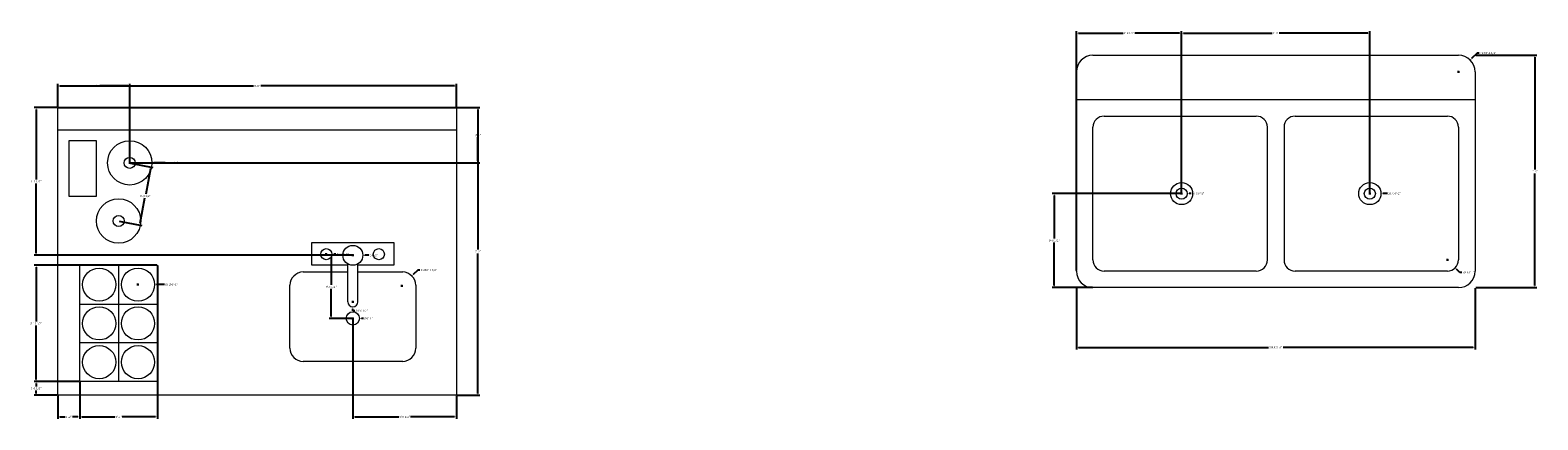
# Model space of a CAD drawing. Units: inches. Extents: x 226 to 1155, y 22 to 494.
# Tile 4 of 7: x 884 to 1020, y 56 to 91. Entities that reach past the tile are written whole.
import ezdxf

# ---------------------------------------------------------------- set-up
doc = ezdxf.new("R2010")
doc.units = ezdxf.units.IN
doc.header["$MEASUREMENT"] = 0
for name, color, linetype, lineweight in [('A-ANNO-DIMS', 2, 'Continuous', 18), ('A-EQPM', 8, 'Continuous', 18), ('A-FLOR-FIXT', 9, 'Continuous', 18)]:
    doc.layers.add(name, color=color, linetype=linetype, lineweight=lineweight)
doc.styles.get("Standard").update_dxf_attribs({"font": 'arial.ttf'})
doc.dimstyles.get("Standard").update_dxf_attribs({"dimtxt": 0.18, "dimasz": 0.18, "dimexe": 0.18, "dimexo": 0.0625, "dimgap": 0.09, "dimtad": 0, "dimtih": 1, "dimtoh": 1, "dimdec": 4, "dimzin": 0, "dimdsep": 46, "dimlunit": 4, "dimtxsty": 'Standard', "dimcen": 0.09, "dimadec": 0, "dimazin": 0, "dimtfac": 1, "dimtdec": 4, "dimtofl": 0, "dimtmove": 0, "dimatfit": 3, "dimfxl": 1, "dimtolj": 1, "dimtzin": 0, "dimarcsym": 0})

# ---------------------------------------------------------------- blocks, each defined once
blk = doc.blocks.new('Sink-double - 36 in top')
for p, q in [((-18, -4), (18, -4)), ((-0.75, -18.5), (-0.75, -6.5)), ((0.75, -6.5), (0.75, -18.5))]:
    blk.add_line(p, q)
for points in [[(-16.5, 0), (16.5, 0)], [(-18, -19.5), (-18, -1.5)], [(18, -1.5), (18, -19.5)], [(-16.5, -18.5), (-16.5, -6.5)], [(-15.5, -5.5), (-1.75, -5.5)], [(1.75, -5.5), (15.5, -5.5)], [(16.5, -6.5), (16.5, -18.5)], [(-1.75, -19.5), (-15.5, -19.5)], [(15.5, -19.5), (1.75, -19.5)], [(16.5, -21), (-16.5, -21)]]:
    blk.add_lwpolyline(points)
for centre, radius in [((-8.5, -12.5), 1), ((-8.5, -12.5), 0.5), ((8.5, -12.5), 1), ((8.5, -12.5), 0.5)]:
    blk.add_circle(centre, radius)
for centre, radius, start, end in [((-16.5, -1.5), 1.5, 90, 180), ((16.5, -1.5), 1.5, 0, 90), ((-15.5, -6.5), 1, 90, 180), ((-1.75, -6.5), 1, 0, 90), ((1.75, -6.5), 1, 90, 180), ((15.5, -6.5), 1, 0, 90), ((-15.5, -18.5), 1, 180, 270), ((-1.75, -18.5), 1, 270, 0), ((1.75, -18.5), 1, 180, 270), ((15.5, -18.5), 1, 270, 0), ((-16.5, -19.5), 1.5, 180, 270), ((16.5, -19.5), 1.5, 270, 0)]:
    blk.add_arc(centre, radius, start, end)
blk = doc.blocks.new('*D52')
at = {"layer": 'A-ANNO-DIMS', "color": 0, "lineweight": -2, "transparency": 16777216}
for p, q in [((978, 67.6), (978, 62.08)), ((1014, 67.6), (1014, 62.08)), ((978.18, 62.26), (995.34, 62.26)), ((1013.82, 62.26), (996.66, 62.26))]:
    blk.add_line(p, q, dxfattribs=at)
at = {"layer": 'A-ANNO-DIMS', "color": 0, "transparency": 16777216}
for points in [[(978.18, 62.29), (978.18, 62.23), (978, 62.26)], [(1013.82, 62.29), (1013.82, 62.23), (1014, 62.26)]]:
    blk.add_solid(points, dxfattribs=at)
at = {"layer": 'Defpoints', "color": 0, "transparency": 16777216}
for p in [(978, 67.66), (1014, 67.66), (1014, 62.26)]:
    blk.add_point(p, dxfattribs=at)
at = {"layer": 'A-ANNO-DIMS', "color": 0, "transparency": 16777216, "insert": (996, 62.26), "char_height": 0.18, "attachment_point": 5}
blk.add_mtext('\\A1;SINK 3\'-0"', dxfattribs=at)
blk = doc.blocks.new('*D53')
at = {"layer": 'A-ANNO-DIMS', "color": 0, "lineweight": -2, "transparency": 16777216}
for p, q in [((1014.06, 88.66), (1019.58, 88.66)), ((1019.4, 88.48), (1019.4, 78.34)), ((1019.4, 67.84), (1019.4, 77.98)), ((1014.06, 67.66), (1019.58, 67.66))]:
    blk.add_line(p, q, dxfattribs=at)
at = {"layer": 'A-ANNO-DIMS', "color": 0, "transparency": 16777216}
for points in [[(1019.37, 88.48), (1019.43, 88.48), (1019.4, 88.66)], [(1019.37, 67.84), (1019.43, 67.84), (1019.4, 67.66)]]:
    blk.add_solid(points, dxfattribs=at)
at = {"layer": 'Defpoints', "color": 0, "transparency": 16777216}
for p in [(1014, 88.66), (1019.4, 88.66), (1014, 67.66)]:
    blk.add_point(p, dxfattribs=at)
at = {"layer": 'A-ANNO-DIMS', "color": 0, "transparency": 16777216, "insert": (1019.4, 78.16), "char_height": 0.18, "attachment_point": 5}
blk.add_mtext('\\A1;1\'-9"', dxfattribs=at)
blk = doc.blocks.new('*D104')
at = {"layer": 'A-ANNO-DIMS', "color": 0, "lineweight": -2, "transparency": 16777216}
for p, q in [((978, 69.22), (978, 90.84)), ((978.18, 90.66), (982.21, 90.66)), ((987.32, 90.66), (983.29, 90.66)), ((987.5, 76.22), (987.5, 90.84))]:
    blk.add_line(p, q, dxfattribs=at)
at = {"layer": 'A-ANNO-DIMS', "color": 0, "transparency": 16777216}
for points in [[(978.18, 90.69), (978.18, 90.63), (978, 90.66)], [(987.32, 90.69), (987.32, 90.63), (987.5, 90.66)]]:
    blk.add_solid(points, dxfattribs=at)
at = {"layer": 'Defpoints', "color": 0, "transparency": 16777216}
for p in [(987.5, 90.66), (987.5, 76.16), (978, 69.16)]:
    blk.add_point(p, dxfattribs=at)
at = {"layer": 'A-ANNO-DIMS', "color": 0, "transparency": 16777216, "insert": (982.75, 90.66), "char_height": 0.18, "attachment_point": 5}
blk.add_mtext('\\A1;0\'-9 1/2"', dxfattribs=at)
blk = doc.blocks.new('*D105')
at = {"layer": 'A-ANNO-DIMS', "color": 0, "lineweight": -2, "transparency": 16777216}
for p, q in [((987.5, 76.22), (987.5, 90.84)), ((987.68, 90.66), (995.68, 90.66)), ((1004.32, 90.66), (996.32, 90.66)), ((1004.5, 76.22), (1004.5, 90.84))]:
    blk.add_line(p, q, dxfattribs=at)
at = {"layer": 'A-ANNO-DIMS', "color": 0, "transparency": 16777216}
for points in [[(987.68, 90.69), (987.68, 90.63), (987.5, 90.66)], [(1004.32, 90.69), (1004.32, 90.63), (1004.5, 90.66)]]:
    blk.add_solid(points, dxfattribs=at)
at = {"layer": 'Defpoints', "color": 0, "transparency": 16777216}
for p in [(1004.5, 90.66), (987.5, 76.16), (1004.5, 76.16)]:
    blk.add_point(p, dxfattribs=at)
at = {"layer": 'A-ANNO-DIMS', "color": 0, "transparency": 16777216, "insert": (996, 90.66), "char_height": 0.18, "attachment_point": 5}
blk.add_mtext('\\A1;1\'-5"', dxfattribs=at)
blk = doc.blocks.new('*D106')
at = {"layer": 'A-ANNO-DIMS', "color": 0, "lineweight": -2, "transparency": 16777216}
for p, q in [((987.44, 76.16), (975.82, 76.16)), ((976, 75.98), (976, 72.09)), ((976, 67.84), (976, 71.73)), ((979.44, 67.66), (975.82, 67.66))]:
    blk.add_line(p, q, dxfattribs=at)
at = {"layer": 'A-ANNO-DIMS', "color": 0, "transparency": 16777216}
for points in [[(975.97, 75.98), (976.03, 75.98), (976, 76.16)], [(975.97, 67.84), (976.03, 67.84), (976, 67.66)]]:
    blk.add_solid(points, dxfattribs=at)
at = {"layer": 'Defpoints', "color": 0, "transparency": 16777216}
for p in [(976, 76.16), (987.5, 76.16), (979.5, 67.66)]:
    blk.add_point(p, dxfattribs=at)
at = {"layer": 'A-ANNO-DIMS', "color": 0, "transparency": 16777216, "insert": (976, 71.91), "char_height": 0.18, "attachment_point": 5}
blk.add_mtext('\\A1;0\'-8 1/2"', dxfattribs=at)
blk = doc.blocks.new('*D107')
at = {"layer": 'A-ANNO-DIMS', "color": 0, "lineweight": -2, "transparency": 16777216}
for p, q in [((886.01, 83.99), (886.01, 86.06)), ((886.19, 85.88), (903.68, 85.88)), ((921.83, 85.88), (904.34, 85.88)), ((922.01, 83.99), (922.01, 86.06))]:
    blk.add_line(p, q, dxfattribs=at)
at = {"layer": 'A-ANNO-DIMS', "color": 0, "transparency": 16777216}
for points in [[(886.19, 85.91), (886.19, 85.85), (886.01, 85.88)], [(921.83, 85.91), (921.83, 85.85), (922.01, 85.88)]]:
    blk.add_solid(points, dxfattribs=at)
at = {"layer": 'Defpoints', "color": 0, "transparency": 16777216}
for p in [(922.01, 85.88), (886.01, 83.93), (922.01, 83.93)]:
    blk.add_point(p, dxfattribs=at)
at = {"layer": 'A-ANNO-DIMS', "color": 0, "transparency": 16777216, "insert": (904.01, 85.88), "char_height": 0.18, "attachment_point": 5}
blk.add_mtext('\\A1;3\'-0"', dxfattribs=at)
blk = doc.blocks.new('*D108')
at = {"layer": 'A-ANNO-DIMS', "color": 0, "lineweight": -2, "transparency": 16777216}
for p, q in [((922.07, 83.93), (924.14, 83.93)), ((923.96, 83.75), (923.96, 71.11)), ((923.96, 58.11), (923.96, 70.75)), ((922.07, 57.93), (924.14, 57.93))]:
    blk.add_line(p, q, dxfattribs=at)
at = {"layer": 'A-ANNO-DIMS', "color": 0, "transparency": 16777216}
for points in [[(923.93, 83.75), (923.99, 83.75), (923.96, 83.93)], [(923.93, 58.11), (923.99, 58.11), (923.96, 57.93)]]:
    blk.add_solid(points, dxfattribs=at)
at = {"layer": 'Defpoints', "color": 0, "transparency": 16777216}
for p in [(922.01, 83.93), (923.96, 83.93), (922.01, 57.93)]:
    blk.add_point(p, dxfattribs=at)
at = {"layer": 'A-ANNO-DIMS', "color": 0, "transparency": 16777216, "insert": (923.96, 70.93), "char_height": 0.18, "attachment_point": 5}
blk.add_mtext('\\A1;2\'-2"', dxfattribs=at)
blk = doc.blocks.new('*D109')
at = {"layer": 'A-ANNO-DIMS', "color": 0, "lineweight": -2, "transparency": 16777216}
for p, q in [((888.01, 59.12), (888.01, 55.8)), ((886.01, 57.87), (886.01, 55.8)), ((886.19, 55.98), (886.68, 55.98)), ((887.83, 55.98), (887.34, 55.98))]:
    blk.add_line(p, q, dxfattribs=at)
at = {"layer": 'A-ANNO-DIMS', "color": 0, "transparency": 16777216}
for points in [[(886.19, 56.01), (886.19, 55.95), (886.01, 55.98)], [(887.83, 56.01), (887.83, 55.95), (888.01, 55.98)]]:
    blk.add_solid(points, dxfattribs=at)
at = {"layer": 'Defpoints', "color": 0, "transparency": 16777216}
for p in [(888.01, 59.18), (886.01, 57.93), (888.01, 55.98)]:
    blk.add_point(p, dxfattribs=at)
at = {"layer": 'A-ANNO-DIMS', "color": 0, "transparency": 16777216, "insert": (887.01, 55.98), "char_height": 0.18, "attachment_point": 5}
blk.add_mtext('\\A1;0\'-2"', dxfattribs=at)
blk = doc.blocks.new('*D110')
at = {"layer": 'A-ANNO-DIMS', "color": 0, "lineweight": -2, "transparency": 16777216}
for p, q in [((887.95, 59.18), (883.88, 59.18)), ((884.06, 59), (884.06, 58.74)), ((885.95, 57.93), (883.88, 57.93)), ((884.06, 58.11), (884.06, 58.37))]:
    blk.add_line(p, q, dxfattribs=at)
at = {"layer": 'A-ANNO-DIMS', "color": 0, "transparency": 16777216}
for points in [[(884.03, 59), (884.09, 59), (884.06, 59.18)], [(884.03, 58.11), (884.09, 58.11), (884.06, 57.93)]]:
    blk.add_solid(points, dxfattribs=at)
at = {"layer": 'Defpoints', "color": 0, "transparency": 16777216}
for p in [(884.06, 59.18), (888.01, 59.18), (886.01, 57.93)]:
    blk.add_point(p, dxfattribs=at)
at = {"layer": 'A-ANNO-DIMS', "color": 0, "transparency": 16777216, "insert": (884.06, 58.56), "char_height": 0.18, "attachment_point": 5}
blk.add_mtext('\\A1;0\'-1 1/2"', dxfattribs=at)
blk = doc.blocks.new('*D111')
at = {"layer": 'A-ANNO-DIMS', "color": 0, "lineweight": -2, "transparency": 16777216}
for p, q in [((895.01, 69.62), (895.01, 55.8)), ((888.01, 59.12), (888.01, 55.8)), ((888.19, 55.98), (891.18, 55.98)), ((894.83, 55.98), (891.84, 55.98))]:
    blk.add_line(p, q, dxfattribs=at)
at = {"layer": 'A-ANNO-DIMS', "color": 0, "transparency": 16777216}
for points in [[(888.19, 56.01), (888.19, 55.95), (888.01, 55.98)], [(894.83, 56.01), (894.83, 55.95), (895.01, 55.98)]]:
    blk.add_solid(points, dxfattribs=at)
at = {"layer": 'Defpoints', "color": 0, "transparency": 16777216}
for p in [(895.01, 69.68), (888.01, 59.18), (895.01, 55.98)]:
    blk.add_point(p, dxfattribs=at)
at = {"layer": 'A-ANNO-DIMS', "color": 0, "transparency": 16777216, "insert": (891.51, 55.98), "char_height": 0.18, "attachment_point": 5}
blk.add_mtext('\\A1;0\'-7"', dxfattribs=at)
blk = doc.blocks.new('*D112')
at = {"layer": 'A-ANNO-DIMS', "color": 0, "lineweight": -2, "transparency": 16777216}
for p, q in [((894.95, 69.68), (883.88, 69.68)), ((884.06, 69.5), (884.06, 64.61)), ((884.06, 59.36), (884.06, 64.25)), ((887.95, 59.18), (883.88, 59.18))]:
    blk.add_line(p, q, dxfattribs=at)
at = {"layer": 'A-ANNO-DIMS', "color": 0, "transparency": 16777216}
for points in [[(884.03, 69.5), (884.09, 69.5), (884.06, 69.68)], [(884.03, 59.36), (884.09, 59.36), (884.06, 59.18)]]:
    blk.add_solid(points, dxfattribs=at)
at = {"layer": 'Defpoints', "color": 0, "transparency": 16777216}
for p in [(884.06, 69.68), (895.01, 69.68), (888.01, 59.18)]:
    blk.add_point(p, dxfattribs=at)
at = {"layer": 'A-ANNO-DIMS', "color": 0, "transparency": 16777216, "insert": (884.06, 64.43), "char_height": 0.18, "attachment_point": 5}
blk.add_mtext('\\A1;0\'-10 1/2"', dxfattribs=at)
blk = doc.blocks.new('*D113')
at = {"layer": 'A-ANNO-DIMS', "color": 0, "lineweight": -2, "transparency": 16777216}
for p, q in [((912.66, 64.82), (912.66, 55.8)), ((922.01, 57.87), (922.01, 55.8)), ((912.84, 55.98), (916.8, 55.98)), ((921.83, 55.98), (917.88, 55.98))]:
    blk.add_line(p, q, dxfattribs=at)
at = {"layer": 'A-ANNO-DIMS', "color": 0, "transparency": 16777216}
for points in [[(912.84, 56.01), (912.84, 55.95), (912.66, 55.98)], [(921.83, 56.01), (921.83, 55.95), (922.01, 55.98)]]:
    blk.add_solid(points, dxfattribs=at)
at = {"layer": 'Defpoints', "color": 0, "transparency": 16777216}
for p in [(912.66, 64.88), (922.01, 57.93), (912.66, 55.98)]:
    blk.add_point(p, dxfattribs=at)
at = {"layer": 'A-ANNO-DIMS', "color": 0, "transparency": 16777216, "insert": (917.34, 55.98), "char_height": 0.18, "attachment_point": 5}
blk.add_mtext('\\A1;0\'-9 1/2"', dxfattribs=at)
blk = doc.blocks.new('*D114')
at = {"layer": 'A-ANNO-DIMS', "color": 0, "lineweight": -2, "transparency": 16777216}
for p, q in [((885.95, 83.93), (883.88, 83.93)), ((884.06, 83.75), (884.06, 77.44)), ((884.06, 70.76), (884.06, 77.07)), ((912.6, 70.58), (883.88, 70.58))]:
    blk.add_line(p, q, dxfattribs=at)
at = {"layer": 'A-ANNO-DIMS', "color": 0, "transparency": 16777216}
for points in [[(884.03, 83.75), (884.09, 83.75), (884.06, 83.93)], [(884.03, 70.76), (884.09, 70.76), (884.06, 70.58)]]:
    blk.add_solid(points, dxfattribs=at)
at = {"layer": 'Defpoints', "color": 0, "transparency": 16777216}
for p in [(886.01, 83.93), (884.06, 70.58), (912.66, 70.58)]:
    blk.add_point(p, dxfattribs=at)
at = {"layer": 'A-ANNO-DIMS', "color": 0, "transparency": 16777216, "insert": (884.06, 77.26), "char_height": 0.18, "attachment_point": 5}
blk.add_mtext('\\A1;1\'-1 1/2"', dxfattribs=at)
blk = doc.blocks.new('*D115')
at = {"layer": 'A-ANNO-DIMS', "color": 0, "lineweight": -2, "transparency": 16777216}
for p, q in [((912.6, 70.58), (910.53, 70.58)), ((910.71, 70.4), (910.71, 67.91)), ((910.71, 65.06), (910.71, 67.55)), ((912.6, 64.88), (910.53, 64.88))]:
    blk.add_line(p, q, dxfattribs=at)
at = {"layer": 'A-ANNO-DIMS', "color": 0, "transparency": 16777216}
for points in [[(910.68, 70.4), (910.74, 70.4), (910.71, 70.58)], [(910.68, 65.06), (910.74, 65.06), (910.71, 64.88)]]:
    blk.add_solid(points, dxfattribs=at)
at = {"layer": 'Defpoints', "color": 0, "transparency": 16777216}
for p in [(910.71, 70.58), (912.66, 70.58), (912.66, 64.88)]:
    blk.add_point(p, dxfattribs=at)
at = {"layer": 'A-ANNO-DIMS', "color": 0, "transparency": 16777216, "insert": (910.71, 67.73), "char_height": 0.18, "attachment_point": 5}
blk.add_mtext('\\A1;0\'-5 1/2"', dxfattribs=at)
blk = doc.blocks.new('*D116')
at = {"layer": 'A-ANNO-DIMS', "color": 0, "lineweight": -2, "transparency": 16777216}
for p, q in [((886.01, 83.99), (886.01, 86.06)), ((886.19, 85.88), (888.72, 85.88)), ((892.33, 85.88), (889.8, 85.88)), ((892.51, 78.99), (892.51, 86.06))]:
    blk.add_line(p, q, dxfattribs=at)
at = {"layer": 'A-ANNO-DIMS', "color": 0, "transparency": 16777216}
for points in [[(886.19, 85.91), (886.19, 85.85), (886.01, 85.88)], [(892.33, 85.91), (892.33, 85.85), (892.51, 85.88)]]:
    blk.add_solid(points, dxfattribs=at)
at = {"layer": 'Defpoints', "color": 0, "transparency": 16777216}
for p in [(892.51, 85.88), (886.01, 83.93), (892.51, 78.93)]:
    blk.add_point(p, dxfattribs=at)
at = {"layer": 'A-ANNO-DIMS', "color": 0, "transparency": 16777216, "insert": (889.26, 85.88), "char_height": 0.18, "attachment_point": 5}
blk.add_mtext('\\A1;0\'-6 1/2"', dxfattribs=at)
blk = doc.blocks.new('*D117')
at = {"layer": 'A-ANNO-DIMS', "color": 0, "lineweight": -2, "transparency": 16777216}
for p, q in [((886.07, 83.93), (924.14, 83.93)), ((923.96, 83.75), (923.96, 81.61)), ((923.96, 79.11), (923.96, 81.25)), ((892.57, 78.93), (924.14, 78.93))]:
    blk.add_line(p, q, dxfattribs=at)
at = {"layer": 'A-ANNO-DIMS', "color": 0, "transparency": 16777216}
for points in [[(923.93, 83.75), (923.99, 83.75), (923.96, 83.93)], [(923.93, 79.11), (923.99, 79.11), (923.96, 78.93)]]:
    blk.add_solid(points, dxfattribs=at)
at = {"layer": 'Defpoints', "color": 0, "transparency": 16777216}
for p in [(886.01, 83.93), (892.51, 78.93), (923.96, 78.93)]:
    blk.add_point(p, dxfattribs=at)
at = {"layer": 'A-ANNO-DIMS', "color": 0, "transparency": 16777216, "insert": (923.96, 81.43), "char_height": 0.18, "attachment_point": 5}
blk.add_mtext('\\A1;0\'-5"', dxfattribs=at)
blk = doc.blocks.new('*D118')
at = {"layer": 'A-ANNO-DIMS', "color": 0, "lineweight": -2, "transparency": 16777216}
for p, q in [((892.57, 78.92), (894.6, 78.53)), ((894.39, 78.39), (893.96, 76.12)), ((893.46, 73.49), (893.89, 75.76)), ((891.57, 73.67), (893.6, 73.28))]:
    blk.add_line(p, q, dxfattribs=at)
at = {"layer": 'A-ANNO-DIMS', "color": 0, "transparency": 16777216}
for points in [[(894.36, 78.4), (894.42, 78.38), (894.43, 78.57)], [(893.43, 73.5), (893.49, 73.49), (893.43, 73.32)]]:
    blk.add_solid(points, dxfattribs=at)
at = {"layer": 'Defpoints', "color": 0, "transparency": 16777216}
for p in [(892.51, 78.93), (891.51, 73.68), (893.43, 73.32)]:
    blk.add_point(p, dxfattribs=at)
at = {"layer": 'A-ANNO-DIMS', "color": 0, "transparency": 16777216, "insert": (893.93, 75.94), "char_height": 0.18, "attachment_point": 5}
blk.add_mtext('\\A1;0\'-5 1/2"', dxfattribs=at)
blk = doc.blocks.new('*D127')
at = {"layer": 'A-ANNO-DIMS', "color": 0, "lineweight": -2, "transparency": 16777216}
for p, q in [((1014.2, 88.86), (1013.69, 88.35)), ((1014.38, 88.86), (1014.2, 88.86)), ((1012.41, 87.16), (1012.59, 87.16)), ((1012.5, 87.07), (1012.5, 87.25))]:
    blk.add_line(p, q, dxfattribs=at)
at = {"layer": 'A-ANNO-DIMS', "color": 0, "transparency": 16777216}
blk.add_solid([(1013.66, 88.37), (1013.71, 88.32), (1013.56, 88.22)], dxfattribs=at)
at = {"layer": 'Defpoints', "color": 0, "transparency": 16777216}
for p in [(1012.5, 87.16), (1013.56, 88.22)]:
    blk.add_point(p, dxfattribs=at)
at = {"layer": 'A-ANNO-DIMS', "color": 0, "transparency": 16777216, "insert": (1015.2, 88.86), "char_height": 0.18, "attachment_point": 5}
blk.add_mtext('\\A1;4X R0\'-1 1/2"', dxfattribs=at)
blk = doc.blocks.new('*D128')
at = {"layer": 'A-ANNO-DIMS', "color": 0, "lineweight": -2, "transparency": 16777216}
for p, q in [((1011.41, 70.16), (1011.59, 70.16)), ((1011.5, 70.07), (1011.5, 70.25)), ((1012.63, 69.03), (1012.33, 69.32)), ((1012.81, 69.03), (1012.63, 69.03))]:
    blk.add_line(p, q, dxfattribs=at)
at = {"layer": 'A-ANNO-DIMS', "color": 0, "transparency": 16777216}
blk.add_solid([(1012.35, 69.35), (1012.31, 69.3), (1012.2, 69.45)], dxfattribs=at)
at = {"layer": 'Defpoints', "color": 0, "transparency": 16777216}
for p in [(1011.5, 70.16), (1012.2, 69.45)]:
    blk.add_point(p, dxfattribs=at)
at = {"layer": 'A-ANNO-DIMS', "color": 0, "transparency": 16777216, "insert": (1013.42, 69.03), "char_height": 0.18, "attachment_point": 5}
blk.add_mtext('\\A1;8X R0\'-1"', dxfattribs=at)
blk = doc.blocks.new('*D129')
at = {"layer": 'A-ANNO-DIMS', "color": 0, "lineweight": -2, "transparency": 16777216}
for p, q in [((1004.5, 76.07), (1004.5, 76.25)), ((1004.41, 76.16), (1004.59, 76.16)), ((1006.1, 76.16), (1005.68, 76.16))]:
    blk.add_line(p, q, dxfattribs=at)
at = {"layer": 'A-ANNO-DIMS', "color": 0, "transparency": 16777216}
blk.add_solid([(1005.68, 76.19), (1005.68, 76.13), (1005.5, 76.16)], dxfattribs=at)
at = {"layer": 'Defpoints', "color": 0, "transparency": 16777216}
for p in [(1003.5, 76.16), (1005.5, 76.16)]:
    blk.add_point(p, dxfattribs=at)
at = {"layer": 'A-ANNO-DIMS', "color": 0, "transparency": 16777216, "insert": (1006.72, 76.16), "char_height": 0.18, "attachment_point": 5}
blk.add_mtext('\\A1;2X ∅0\'-2"', dxfattribs=at)
blk = doc.blocks.new('*D130')
at = {"layer": 'A-ANNO-DIMS', "color": 0, "lineweight": -2, "transparency": 16777216}
for p, q in [((987.5, 76.07), (987.5, 76.25)), ((987.41, 76.16), (987.59, 76.16)), ((988.36, 76.16), (988.18, 76.16))]:
    blk.add_line(p, q, dxfattribs=at)
at = {"layer": 'A-ANNO-DIMS', "color": 0, "transparency": 16777216}
blk.add_solid([(988.18, 76.19), (988.18, 76.13), (988, 76.16)], dxfattribs=at)
at = {"layer": 'Defpoints', "color": 0, "transparency": 16777216}
for p in [(987, 76.16), (988, 76.16)]:
    blk.add_point(p, dxfattribs=at)
at = {"layer": 'A-ANNO-DIMS', "color": 0, "transparency": 16777216, "insert": (988.98, 76.16), "char_height": 0.18, "attachment_point": 5}
blk.add_mtext('\\A1;2X ∅0\'-1"', dxfattribs=at)
blk = doc.blocks.new('*D131')
at = {"layer": 'A-ANNO-DIMS', "color": 0, "lineweight": -2, "transparency": 16777216}
for p, q in [((892.51, 78.84), (892.51, 79.02)), ((892.42, 78.93), (892.6, 78.93)), ((895.71, 78.93), (894.69, 78.93))]:
    blk.add_line(p, q, dxfattribs=at)
at = {"layer": 'A-ANNO-DIMS', "color": 0, "transparency": 16777216}
blk.add_solid([(894.69, 78.96), (894.69, 78.9), (894.51, 78.93)], dxfattribs=at)
at = {"layer": 'Defpoints', "color": 0, "transparency": 16777216}
for p in [(890.51, 78.93), (894.51, 78.93)]:
    blk.add_point(p, dxfattribs=at)
at = {"layer": 'A-ANNO-DIMS', "color": 0, "transparency": 16777216, "insert": (896.33, 78.93), "char_height": 0.18, "attachment_point": 5}
blk.add_mtext('\\A1;2X ∅0\'-4"', dxfattribs=at)
blk = doc.blocks.new('*D132')
at = {"layer": 'A-ANNO-DIMS', "color": 0, "lineweight": -2, "transparency": 16777216}
for p, q in [((893.17, 67.93), (893.35, 67.93)), ((893.26, 67.84), (893.26, 68.02)), ((895.66, 67.93), (894.94, 67.93))]:
    blk.add_line(p, q, dxfattribs=at)
at = {"layer": 'A-ANNO-DIMS', "color": 0, "transparency": 16777216}
blk.add_solid([(894.94, 67.96), (894.94, 67.9), (894.76, 67.93)], dxfattribs=at)
at = {"layer": 'Defpoints', "color": 0, "transparency": 16777216}
for p in [(891.76, 67.93), (894.76, 67.93)]:
    blk.add_point(p, dxfattribs=at)
at = {"layer": 'A-ANNO-DIMS', "color": 0, "transparency": 16777216, "insert": (896.28, 67.93), "char_height": 0.18, "attachment_point": 5}
blk.add_mtext('\\A1;6X ∅0\'-3"', dxfattribs=at)
blk = doc.blocks.new('*D133')
at = {"layer": 'A-ANNO-DIMS', "color": 0, "lineweight": -2, "transparency": 16777216}
for p, q in [((918.53, 69.25), (918.12, 68.84)), ((918.71, 69.25), (918.53, 69.25)), ((917, 67.81), (917.18, 67.81)), ((917.09, 67.72), (917.09, 67.9))]:
    blk.add_line(p, q, dxfattribs=at)
at = {"layer": 'A-ANNO-DIMS', "color": 0, "transparency": 16777216}
blk.add_solid([(918.1, 68.86), (918.14, 68.82), (917.99, 68.71)], dxfattribs=at)
at = {"layer": 'Defpoints', "color": 0, "transparency": 16777216}
for p in [(917.99, 68.71), (917.09, 67.81)]:
    blk.add_point(p, dxfattribs=at)
at = {"layer": 'A-ANNO-DIMS', "color": 0, "transparency": 16777216, "insert": (919.53, 69.25), "char_height": 0.18, "attachment_point": 5}
blk.add_mtext('\\A1;4X R0\'-1 1/2"', dxfattribs=at)
blk = doc.blocks.new('*D134')
at = {"layer": 'A-ANNO-DIMS', "color": 0, "lineweight": -2, "transparency": 16777216}
for p, q in [((912.57, 70.58), (912.75, 70.58)), ((912.66, 70.49), (912.66, 70.67)), ((914.1, 70.58), (913.74, 70.58))]:
    blk.add_line(p, q, dxfattribs=at)
at = {"layer": 'A-ANNO-DIMS', "color": 0, "transparency": 16777216}
blk.add_solid([(913.74, 70.61), (913.74, 70.55), (913.56, 70.58)], dxfattribs=at)
at = {"layer": 'Defpoints', "color": 0, "transparency": 16777216}
for p in [(911.76, 70.58), (913.56, 70.58)]:
    blk.add_point(p, dxfattribs=at)
at = {"layer": 'A-ANNO-DIMS', "color": 0, "transparency": 16777216, "insert": (914.53, 70.58), "char_height": 0.18, "attachment_point": 5}
blk.add_mtext('\\A1;∅0\'-2"', dxfattribs=at)
blk = doc.blocks.new('*D135')
at = {"layer": 'A-ANNO-DIMS', "color": 0, "lineweight": -2, "transparency": 16777216}
for p, q in [((912.57, 64.88), (912.75, 64.88)), ((912.66, 64.79), (912.66, 64.97)), ((913.62, 64.88), (913.44, 64.88))]:
    blk.add_line(p, q, dxfattribs=at)
at = {"layer": 'A-ANNO-DIMS', "color": 0, "transparency": 16777216}
blk.add_solid([(913.44, 64.91), (913.44, 64.85), (913.26, 64.88)], dxfattribs=at)
at = {"layer": 'Defpoints', "color": 0, "transparency": 16777216}
for p in [(912.06, 64.88), (913.26, 64.88)]:
    blk.add_point(p, dxfattribs=at)
at = {"layer": 'A-ANNO-DIMS', "color": 0, "transparency": 16777216, "insert": (914.05, 64.88), "char_height": 0.18, "attachment_point": 5}
blk.add_mtext('\\A1;∅0\'-1"', dxfattribs=at)
blk = doc.blocks.new('*D136')
at = {"layer": 'A-ANNO-DIMS', "color": 0, "lineweight": -2, "transparency": 16777216}
for p, q in [((910.17, 70.68), (910.35, 70.68)), ((910.26, 70.59), (910.26, 70.77)), ((911.12, 70.68), (910.94, 70.68))]:
    blk.add_line(p, q, dxfattribs=at)
at = {"layer": 'A-ANNO-DIMS', "color": 0, "transparency": 16777216}
blk.add_solid([(910.94, 70.71), (910.94, 70.65), (910.76, 70.68)], dxfattribs=at)
at = {"layer": 'Defpoints', "color": 0, "transparency": 16777216}
for p in [(909.76, 70.68), (910.76, 70.68)]:
    blk.add_point(p, dxfattribs=at)
at = {"layer": 'A-ANNO-DIMS', "color": 0, "transparency": 16777216, "insert": (911.74, 70.68), "char_height": 0.18, "attachment_point": 5}
blk.add_mtext('\\A1;4X ∅0\'-1"', dxfattribs=at)
blk = doc.blocks.new('*D137')
at = {"layer": 'A-ANNO-DIMS', "color": 0, "lineweight": -2, "transparency": 16777216}
for p, q in [((912.57, 66.38), (912.75, 66.38)), ((912.66, 66.29), (912.66, 66.47)), ((912.66, 65.57), (912.66, 65.75)), ((912.84, 65.57), (912.66, 65.57))]:
    blk.add_line(p, q, dxfattribs=at)
at = {"layer": 'A-ANNO-DIMS', "color": 0, "transparency": 16777216}
blk.add_solid([(912.69, 65.75), (912.63, 65.75), (912.66, 65.93)], dxfattribs=at)
at = {"layer": 'Defpoints', "color": 0, "transparency": 16777216}
for p in [(912.66, 66.38), (912.66, 65.93)]:
    blk.add_point(p, dxfattribs=at)
at = {"layer": 'A-ANNO-DIMS', "color": 0, "transparency": 16777216, "insert": (913.47, 65.57), "char_height": 0.18, "attachment_point": 5}
blk.add_mtext('\\A1;R0\'-0 1/2"', dxfattribs=at)

msp = doc.modelspace()

# ---------------------------------------------------------------- linework, layer by layer
at = {"layer": 'A-EQPM'}
for p, q in [((886.0117, 83.93166), (922.0117, 83.93166)), ((886.0117, 57.93166), (886.0117, 83.93166)), ((922.0117, 83.93166), (922.0117, 57.93166)), ((886.0117, 81.93166), (922.0117, 81.93166)), ((889.5117, 80.93166), (887.0117, 80.93166)), ((887.0117, 80.93166), (887.0117, 75.93166)), ((889.5117, 75.93166), (889.5117, 80.93166)), ((887.0117, 75.93166), (889.5117, 75.93166)), ((888.0117, 69.68166), (895.0117, 69.68166)), ((888.0117, 59.18166), (888.0117, 69.68166)), ((891.5117, 69.68166), (891.5117, 59.18166)), ((895.0117, 69.68166), (895.0117, 59.18166)), ((912.2117, 66.38166), (912.2117, 69.80326)), ((913.1118, 66.38166), (913.1118, 69.80326)), ((888.0117, 66.18166), (895.0117, 66.18166)), ((895.0117, 62.68166), (888.0117, 62.68166)), ((895.0117, 59.18166), (888.0117, 59.18166)), ((922.0117, 57.93166), (886.0117, 57.93166))]:
    msp.add_line(p, q, dxfattribs=at)
for points in [[(912.2117, 69.68166), (908.9617, 69.68166), (908.9617, 71.73166), (912.7617, 71.73166)], [(912.7604, 71.73166), (916.3618, 71.73166), (916.3618, 69.68166), (913.1118, 69.68166)], [(908.1617, 69.08166), (912.2117, 69.08166)], [(913.1118, 69.08166), (917.1617, 69.08166)], [(906.9617, 62.18166), (906.9617, 67.88166)], [(918.3618, 67.88166), (918.3618, 62.18166)], [(917.1617, 60.98166), (908.1617, 60.98166)]]:
    msp.add_lwpolyline(points, dxfattribs=at)
for centre, radius in [((892.5117, 78.93166), 2), ((892.5117, 78.93166), 0.5), ((891.5117, 73.68166), 2), ((891.5117, 73.68166), 0.5), ((910.2617, 70.68166), 0.5), ((912.6617, 70.58166), 0.9), ((915.0117, 70.68166), 0.5), ((889.7617, 67.93166), 1.5), ((893.2617, 67.93166), 1.5), ((889.7617, 64.43166), 1.5), ((893.2617, 64.43166), 1.5), ((912.6617, 64.88166), 0.6), ((889.7617, 60.93166), 1.5), ((893.2617, 60.93166), 1.5)]:
    msp.add_circle(centre, radius, dxfattribs=at)
for centre, radius, start, end in [((908.2368, 67.80666), 1.2772, 93.36646, 176.6335), ((917.0867, 67.80666), 1.2772, 3.366461, 86.63354), ((912.6617, 66.38166), 0.45, 180, 0), ((908.2368, 62.25666), 1.2772, 183.3665, 266.6335), ((917.0867, 62.25666), 1.2772, 273.3665, 356.6335)]:
    msp.add_arc(centre, radius, start, end, dxfattribs=at)

# ---------------------------------------------------------------- block references
at = {"layer": 'A-FLOR-FIXT'}
msp.add_blockref('Sink-double - 36 in top', (995.99789, 88.65838), dxfattribs=at)

# ---------------------------------------------------------------- dimensions: what is measured, and where the dimension line sits
at = {"layer": 'A-ANNO-DIMS'}
for base, p1, p2, picture, middle in [((987.49789, 90.65838), (977.99789, 69.15838), (987.49789, 76.15838), '*D104', (982.74789, 90.65838)), ((1004.49789, 90.65838), (987.49789, 76.15838), (1004.49789, 76.15838), '*D105', (995.99789, 90.65838)), ((892.5117, 85.88166), (886.0117, 83.93166), (892.5117, 78.93166), '*D116', (889.2617, 85.88166)), ((922.0117, 85.88166), (886.0117, 83.93166), (922.0117, 83.93166), '*D107', (904.0117, 85.88166)), ((895.0117, 55.98166), (888.0117, 59.18166), (895.0117, 69.68166), '*D111', (891.5117, 55.98166)), ((912.6617, 55.981661), (922.0117, 57.931661), (912.6617, 64.881661), '*D113', (917.3367, 55.981661)), ((888.0117, 55.98166), (886.0117, 57.93166), (888.0117, 59.18166), '*D109', (887.0117, 55.98166))]:
    dim = msp.add_linear_dim(base=base, p1=p1, p2=p2, dimstyle='Standard', override={"dimdec": 1, "dimlfac": 1, "dimrnd": 0, "dimzin": 1, "dimdsep": 46, "dimlunit": 4, "dimfrac": 2}, dxfattribs=at)
    dim.commit()
    dim.dimension.update_dxf_attribs({"geometry": picture, "text_midpoint": middle})
for center, mpoint, text, picture, middle in [((1012.49789, 87.15838), (1013.55879, 88.21879), '4X <>', '*D127', (1015.19743, 88.85504)), ((917.0867, 67.80666), (917.9898, 68.7098), '4X <>', '*D133', (919.53375, 69.25168)), ((1011.49789, 70.15838), (1012.20486, 69.45114), '8X <>', '*D128', (1013.41793, 69.02679))]:
    dim = msp.add_radius_dim(center=center, mpoint=mpoint, text=text, dimstyle='Standard', override={"dimdec": 1, "dimlfac": 1, "dimrnd": 0, "dimzin": 1, "dimdsep": 46, "dimlunit": 4, "dimfrac": 2}, dxfattribs=at)
    dim.commit()
    dim.dimension.update_dxf_attribs({"geometry": picture, "text_midpoint": middle, "dimtype": 164})
for base, p1, p2, angle, picture, middle in [((1019.39789, 88.65838), (1013.99789, 67.65838), (1013.99789, 88.65838), 90, '*D53', (1019.39789, 78.15838)), ((884.0617, 70.581661), (886.0117, 83.931661), (912.6617, 70.581661), 90, '*D114', (884.0617, 77.256661)), ((923.9617, 78.93166), (886.0117, 83.93166), (892.5117, 78.93166), 90, '*D117', (923.9617, 81.43166)), ((923.9617, 83.93166), (922.0117, 57.93166), (922.0117, 83.93166), 90, '*D108', (923.9617, 70.93166)), ((893.42726, 73.31679), (892.5117, 78.93166), (891.5117, 73.68166), 259.2157021, '*D118', (893.92726, 75.94179)), ((975.99789, 76.15838), (979.49789, 67.65838), (987.49789, 76.15838), 90, '*D106', (975.99789, 71.90838)), ((884.0617, 69.68166), (888.0117, 59.18166), (895.0117, 69.68166), 90, '*D112', (884.0617, 64.43166)), ((910.7117, 70.58166), (912.6617, 64.88166), (912.6617, 70.58166), 90, '*D115', (910.7117, 67.73166)), ((884.0617, 59.181661), (886.0117, 57.931661), (888.0117, 59.181661), 90, '*D110', (884.0617, 58.556661))]:
    dim = msp.add_linear_dim(base=base, p1=p1, p2=p2, angle=angle, dimstyle='Standard', override={"dimdec": 1, "dimlfac": 1, "dimrnd": 0, "dimzin": 1, "dimdsep": 46, "dimlunit": 4, "dimfrac": 2}, dxfattribs=at)
    dim.commit()
    dim.dimension.update_dxf_attribs({"geometry": picture, "text_midpoint": middle})
for p1, p2, text, picture, middle in [((890.5117, 78.93132), (894.5117, 78.932), '2X <>', '*D131', (895.7117, 78.9322)), ((986.99789, 76.15875), (987.99789, 76.158), '2X <>', '*D130', (988.35789, 76.15773)), ((1003.49789, 76.15875), (1005.49789, 76.158), '2X <>', '*D129', (1006.09789, 76.15777)), ((909.7617, 70.68132), (910.7617, 70.682), '4X <>', '*D136', (911.1217, 70.68224)), ((891.7617, 67.93132), (894.7617, 67.932), '6X <>', '*D132', (895.6617, 67.9322))]:
    dim = msp.add_diameter_dim_2p(p1=p1, p2=p2, text=text, dimstyle='Standard', override={"dimdec": 1, "dimlfac": 1, "dimrnd": 0, "dimzin": 1, "dimdsep": 46, "dimlunit": 4, "dimfrac": 2}, dxfattribs=at)
    dim.commit()
    dim.dimension.update_dxf_attribs({"geometry": picture, "text_midpoint": middle, "dimtype": 163})
for p1, p2, picture, middle in [((911.7617, 70.58132), (913.5617, 70.582), '*D134', (914.1017, 70.5822)), ((912.0617, 64.88132), (913.2617, 64.882), '*D135', (913.6217, 64.8822))]:
    dim = msp.add_diameter_dim_2p(p1=p1, p2=p2, dimstyle='Standard', override={"dimdec": 1, "dimlfac": 1, "dimrnd": 0, "dimzin": 1, "dimdsep": 46, "dimlunit": 4, "dimfrac": 2}, dxfattribs=at)
    dim.commit()
    dim.dimension.update_dxf_attribs({"geometry": picture, "text_midpoint": middle, "dimtype": 163})
dim = msp.add_linear_dim(base=(1013.99789, 62.25838), p1=(977.99789, 67.65838), p2=(1013.99789, 67.65838), text='SINK <>', dimstyle='Standard', override={"dimdec": 1, "dimlfac": 1, "dimrnd": 0, "dimzin": 1, "dimdsep": 46, "dimlunit": 4, "dimfrac": 2}, dxfattribs=at)
dim.commit()
dim.dimension.update_dxf_attribs({"geometry": '*D52', "text_midpoint": (995.99789, 62.25838)})
dim = msp.add_radius_dim(center=(912.6617, 66.38166), mpoint=(912.662, 65.93166), dimstyle='Standard', override={"dimdec": 1, "dimlfac": 1, "dimrnd": 0, "dimzin": 1, "dimdsep": 46, "dimlunit": 4, "dimfrac": 2}, dxfattribs=at)
dim.commit()
dim.dimension.update_dxf_attribs({"geometry": '*D137', "text_midpoint": (913.46733, 65.57166)})

doc.saveas('drawing.dxf')
